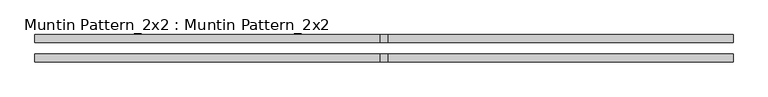
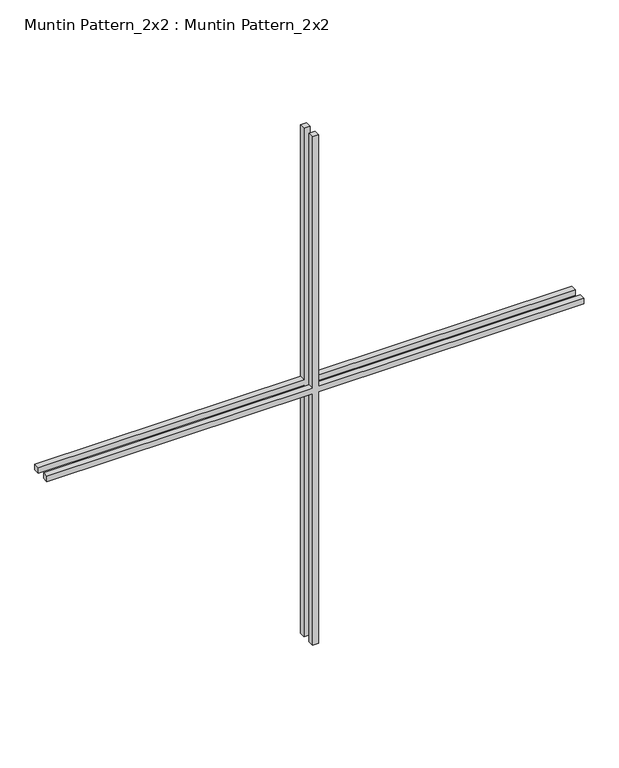
"""IFC4 building model written with IfcOpenShell, lengths in millimetres: proxy geometry, Muntin Pattern_2x2 : Muntin Pattern_2x2."""

from ifc_helpers import new_model, si_unit, frame, origin, place, context, project, spatial, polyline, outline, extrude, source, transform, mapped, element, save


def muntin_pattern_2x2_muntin_pattern_2x2_3e35e312(model_context):
    return source(origin(), model_context, "Body", "SweptSolid", [
        extrude(outline(polyline([(577.85, -6.35), (577.85, -571.5), (565.15, -571.5), (565.15, -6.35), (0.0, -6.35), (0.0, 6.35), (565.15, 6.35), (565.15, 571.5), (577.85, 571.5), (577.85, 6.35), (1143.0, 6.35), (1143.0, -6.35), (577.85, -6.35)])), frame((0.0, -22.225, 0.0), z_axis=(0.0, 1.0, 0.0), x_axis=(0.0, 0.0, 1.0)), (0.0, 0.0, 1.0), 12.7),
        extrude(outline(polyline([(577.85, -6.35), (577.85, -571.5), (565.15, -571.5), (565.15, -6.35), (0.0, -6.35), (0.0, 6.35), (565.15, 6.35), (565.15, 571.5), (577.85, 571.5), (577.85, 6.35), (1143.0, 6.35), (1143.0, -6.35), (577.85, -6.35)])), frame((0.0, 9.525, 0.0), z_axis=(0.0, 1.0, 0.0), x_axis=(0.0, 0.0, 1.0)), (0.0, 0.0, 1.0), 12.7),
    ])


if __name__ == "__main__":
    model = new_model("IFC4")
    model_context = context("Model", 3, world=origin())
    ifc_project = project(units=[si_unit("LENGTHUNIT", "METRE", prefix="MILLI")], contexts=[model_context])
    site = spatial("IfcSite", under=ifc_project)
    building = spatial("IfcBuilding", under=site)
    placement = place(None, origin())
    muntin_pattern_2x2_muntin_pattern_2x2_shape = muntin_pattern_2x2_muntin_pattern_2x2_3e35e312(model_context)
    element("IfcBuildingElementProxy", 1, Name="Muntin Pattern_2x2 : Muntin Pattern_2x2", ObjectType="Muntin Pattern_2x2 : Muntin Pattern_2x2", at=placement, inside=building, context=model_context, shape_type="MappedRepresentation", body=[
        mapped(muntin_pattern_2x2_muntin_pattern_2x2_shape, transform((0.0, 0.0, 0.0), x_axis=(1.0, 0.0, 0.0), y_axis=(0.0, 1.0, 0.0), z_axis=(0.0, 0.0, 1.0))),
    ])
    save(model, "model.ifc")

# Revit data of these elements
# Type "Muntin Pattern_2x2 : Muntin Pattern_2x2"
#   Width [instance default] = 4' - 0"
#   Thickness = 0' - 0 1/2"
#   Height [instance default] = 4' - 0"
#   Distance = 0' - 0 3/4"
#   Interior Material [instance default] = none
#   Exterior Material [instance default] = none
#   Default Elevation = 0
# Element 1 (IfcBuildingElementProxy, "Muntin Pattern_2x2 : Muntin Pattern_2x2")
#   Width = 3' - 9"
#   Height = 3' - 9"
#   Interior Material = Wood - Stained
#   Exterior Material = Clad - White
#   Materials on its faces: "Clad - White", "Wood - Stained"
# Materials
#   "Clad - White": class "Wood", colour RGB 242 242 238, transparency 0, Cost = 0
#   "Wood - Stained": class "Wood", colour RGB 224 178 126, transparency 0, Cost = 0
